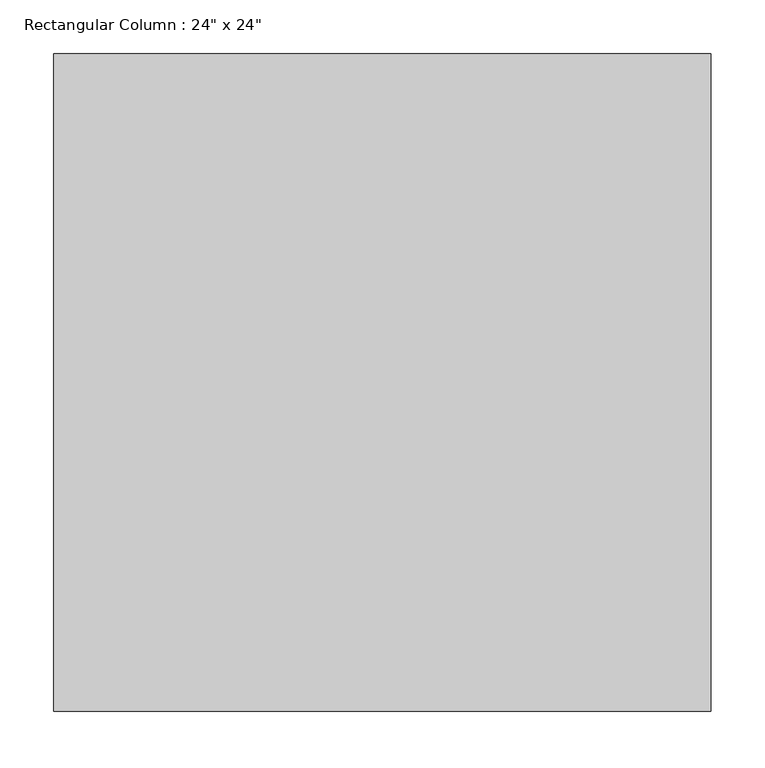
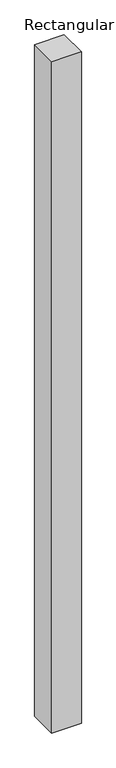
"""IFC4 building model written with IfcOpenShell, lengths in millimetres: column geometry."""

from ifc_helpers import new_model, si_unit, origin, origin_with_axes, place, context, project, spatial, polyline, outline, extrude, source, transform, mapped, element, save


def column_edfe3d85(model_context):
    return source(origin(), model_context, "Body", "SweptSolid", [
        extrude(outline(polyline([(304.8, 304.8), (304.8, -304.8), (-304.8, -304.8), (-304.8, 304.8), (304.8, 304.8)])), origin_with_axes(), (0.0, 0.0, 1.0), 14630.4),
    ])


if __name__ == "__main__":
    model = new_model("IFC4")
    model_context = context("Model", 3, world=origin())
    ifc_project = project(units=[si_unit("LENGTHUNIT", "METRE", prefix="MILLI")], contexts=[model_context])
    site = spatial("IfcSite", under=ifc_project)
    building = spatial("IfcBuilding", under=site)
    placement = place(None, origin())
    column_shape = column_edfe3d85(model_context)
    element("IfcColumn", 1, ObjectType="Rectangular Column : 24\" x 24\"", at=placement, inside=building, context=model_context, shape_type="MappedRepresentation", body=[
        mapped(column_shape, transform((0.0, 0.0, 0.0), x_axis=(1.0, 0.0, 0.0), y_axis=(0.0, 1.0, 0.0), z_axis=(0.0, 0.0, 1.0))),
    ])
    save(model, "model.ifc")

# Revit data of these elements
# Type "Rectangular Column : 24\" x 24\""
#   Assembly Code = "B1010200"
#   Depth = 2' - 0"
#   Offset Base = 0' - 0"
#   Offset Top = 0' - 0"
#   Width = 2' - 0"
#   Material = none
